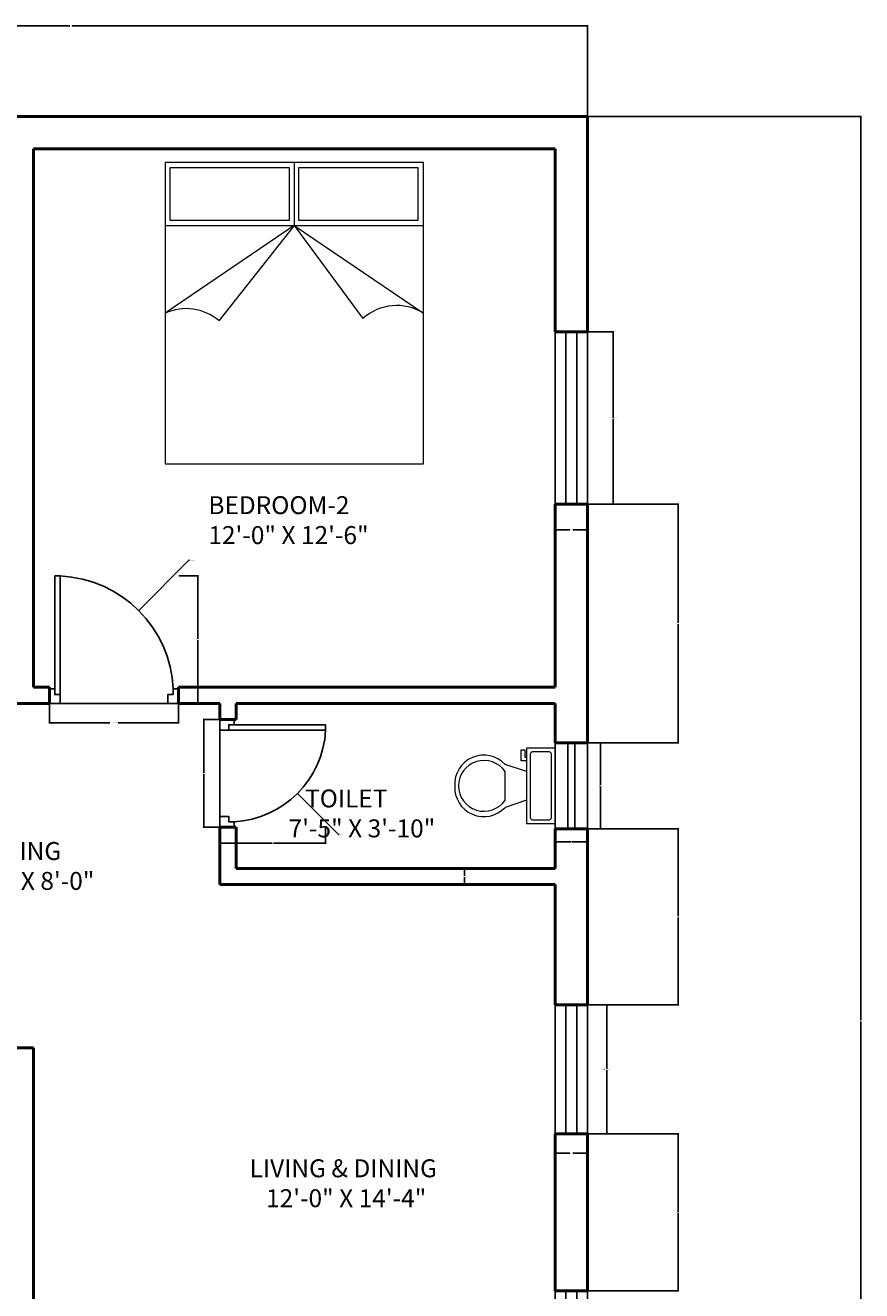
# Model space of a CAD drawing. Units: inches. Extents: x 17078 to 17468, y 5298 to 5853.
# Tile 3 of 3: x 17235 to 17468, y 5500 to 5853. Entities that reach past the tile are written whole.
import ezdxf

# ---------------------------------------------------------------- set-up
doc = ezdxf.new("R2010")
doc.units = ezdxf.units.IN
for name, color, linetype, lineweight in [('A-ANNO-DIMS', 2, 'Continuous', 18), ('A-AREA-IDEN', 7, 'Continuous', 18), ('A-FLOR-FIXT', 9, 'Continuous', 18), ('door', 30, 'Continuous', 25), ('furniture', 9, 'Continuous', 18), ('ventilator', 191, 'Continuous', 25), ('wall', 7, 'Continuous', 50), ('window1', 151, 'Continuous', 25)]:
    doc.layers.add(name, color=color, linetype=linetype, lineweight=lineweight)
doc.styles.get("Standard").update_dxf_attribs({"font": 'arial.ttf'})
doc.dimstyles.get("Standard").update_dxf_attribs({"dimtxt": 0.18, "dimasz": 0.18, "dimexe": 0.18, "dimexo": 0.0625, "dimgap": 0.09, "dimtad": 0, "dimtih": 1, "dimtoh": 1, "dimdec": 4, "dimzin": 0, "dimdsep": 46, "dimtxsty": 'Standard', "dimcen": 0.09, "dimadec": 0, "dimazin": 0, "dimtfac": 1, "dimtdec": 4, "dimtofl": 0, "dimtmove": 0, "dimatfit": 3, "dimfxl": 1, "dimtolj": 1, "dimtzin": 0, "dimarcsym": 0})

# ---------------------------------------------------------------- blocks, each defined once
blk = doc.blocks.new('d1')
at = {"layer": 'door'}
blk.add_line((17631.7, 5593.67), (17667.7, 5593.67), dxfattribs=at)
blk.add_lwpolyline([(17633.2, 5596.17), (17634.7, 5596.17), (17634.7, 5629.17), (17633.2, 5629.17)], close=True, dxfattribs=at)
for points in [[(17634.7, 5593.67), (17631.7, 5593.67), (17631.7, 5597.67), (17633.2, 5597.67), (17633.2, 5596.17), (17634.7, 5596.17), (17634.7, 5593.67)], [(17664.7, 5593.67), (17667.7, 5593.67), (17667.7, 5597.67), (17666.2, 5597.67), (17666.2, 5596.17), (17664.7, 5596.17), (17664.7, 5593.67)]]:
    blk.add_lwpolyline(points, dxfattribs=at)
blk.add_arc((17633.2, 5596.17), 33.03, 2.6026, 87.3974, dxfattribs=at)
blk = doc.blocks.new('d2')
at = {"layer": 'door'}
blk.add_line((17631.7, 5527.56), (17661.7, 5527.56), dxfattribs=at)
blk.add_lwpolyline([(17633.2, 5530.06), (17634.7, 5530.06), (17634.7, 5557.06), (17633.2, 5557.06)], close=True, dxfattribs=at)
for points in [[(17634.7, 5527.56), (17631.7, 5527.56), (17631.7, 5531.56), (17633.2, 5531.56), (17633.2, 5530.06), (17634.7, 5530.06), (17634.7, 5527.56)], [(17658.7, 5527.56), (17661.7, 5527.56), (17661.7, 5531.56), (17660.2, 5531.56), (17660.2, 5530.06), (17658.7, 5530.06), (17658.7, 5527.56)]]:
    blk.add_lwpolyline(points, dxfattribs=at)
blk.add_arc((17633.2, 5530.06), 27.04, 3.1798, 86.8202, dxfattribs=at)
blk = doc.blocks.new('w1')
at = {"layer": 'window1'}
for p, q in [((17477.6, 5616.65), (17477.6, 5580.65)), ((17480.6, 5616.65), (17480.6, 5580.65))]:
    blk.add_line(p, q, dxfattribs=at)
blk.add_lwpolyline([(17474.6, 5580.65), (17483.6, 5580.65), (17483.6, 5616.65), (17474.6, 5616.65)], close=True, dxfattribs=at)
blk = doc.blocks.new('v')
at = {"layer": 'ventilator'}
for p, q in [((17450.03, 5790.51), (17450.03, 5766.51)), ((17452.03, 5790.51), (17452.03, 5766.51))]:
    blk.add_line(p, q, dxfattribs=at)
blk.add_lwpolyline([(17446.53, 5766.51), (17455.53, 5766.51), (17455.53, 5790.51), (17446.53, 5790.51)], close=True, dxfattribs=at)
blk = doc.blocks.new('w2')
at = {"layer": 'window1'}
for p, q in [((17539.72, 5675.98), (17539.72, 5627.98)), ((17542.72, 5675.98), (17542.72, 5627.98))]:
    blk.add_line(p, q, dxfattribs=at)
blk.add_lwpolyline([(17536.72, 5627.98), (17545.72, 5627.98), (17545.72, 5675.98), (17536.72, 5675.98)], close=True, dxfattribs=at)
blk = doc.blocks.new('BED')
at = {"layer": 'furniture'}
for p, q in [((17631.72, 5825.16), (17631.72, 5807.64)), ((17595.72, 5807.64), (17667.72, 5807.64)), ((17631.72, 5807.64), (17595.72, 5783.16)), ((17631.72, 5807.64), (17610.71, 5781.09)), ((17631.72, 5807.64), (17667.72, 5783.16)), ((17631.72, 5807.64), (17650.87, 5781.67))]:
    blk.add_line(p, q, dxfattribs=at)
for points in [[(17595.72, 5741.16), (17667.72, 5741.16), (17667.72, 5825.16), (17595.72, 5825.16)], [(17597.14, 5823.74), (17630.27, 5823.74), (17630.27, 5809), (17597.14, 5809)], [(17633.01, 5823.74), (17666.14, 5823.74), (17666.14, 5809), (17633.01, 5809)]]:
    blk.add_lwpolyline(points, close=True, dxfattribs=at)
for centre, radius, start, end in [((17601.58, 5770.29), 14.15, 49.7949, 114.4561), ((17660.27, 5771.38), 13.94, 57.7012, 132.4176)]:
    blk.add_arc(centre, radius, start, end, dxfattribs=at)
blk = doc.blocks.new('*U8')
for p, q in [((241.3, -152.4), (241.3, -50.8)), ((-254, -215.9), (-203.2, -215.9)), ((-254, -241.3), (-254, -215.9)), ((-177.8, -241.3), (-254, -241.3)), ((-203.2, -215.9), (-203.2, -203.2)), ((-177.8, -203.2), (-177.8, -241.3)), ((-101.6, -203.2), (-152.4, -355.6)), ((101.6, -203.2), (152.4, -355.6)), ((101.6, -355.6), (-101.6, -355.6))]:
    blk.add_line(p, q)
blk.add_lwpolyline([(266.7, -203.2), (266.7, 0), (-266.7, 0), (-266.7, -203.2)], close=True)
for points in [[(-241.3, -50.8), (-241.3, -152.4)], [(215.9, -25.4), (-215.9, -25.4)], [(-215.9, -177.8), (215.9, -177.8)]]:
    blk.add_lwpolyline(points)
for centre, radius, start, end in [((-219.075, -47.625), 22.45064, 81.8699, 188.1301), ((219.075, -47.625), 22.45064, 351.8699, 98.1301), ((-219.075, -155.575), 22.45064, 171.869898, 278.1301), ((219.075, -155.575), 22.45064, 261.8699, 8.1301), ((-12.12088, -505.93752), 205.61935, 133.01722, 273.38), ((0.94996, -504.77674), 181.02486, 124.50543, 269.7), ((-0.94742, -504.77674), 181.02486, 270.3, 55.4946), ((12.12342, -505.93752), 205.61935, 266.62, 46.9828)]:
    blk.add_arc(centre, radius, start, end)
blk = doc.blocks.new('*D9')
at = {"layer": 'A-ANNO-DIMS', "color": 0, "lineweight": -2, "transparency": 16777216}
for p, q in [((17241.53, 5663.96), (17241.53, 5658.44)), ((17277.53, 5663.96), (17277.53, 5658.44)), ((17241.71, 5658.62), (17258.4, 5658.62)), ((17277.35, 5658.62), (17260.67, 5658.62))]:
    blk.add_line(p, q, dxfattribs=at)
at = {"layer": 'A-ANNO-DIMS', "color": 0, "transparency": 16777216}
for points in [[(17241.71, 5658.65), (17241.71, 5658.59), (17241.53, 5658.62)], [(17277.35, 5658.65), (17277.35, 5658.59), (17277.53, 5658.62)]]:
    blk.add_solid(points, dxfattribs=at)
at = {"layer": 'Defpoints', "color": 0, "transparency": 16777216}
for p in [(17241.53, 5664.02), (17277.53, 5664.02), (17277.53, 5658.62)]:
    blk.add_point(p, dxfattribs=at)
at = {"layer": 'A-ANNO-DIMS', "color": 0, "transparency": 16777216, "insert": (17259.53, 5658.62), "char_height": 0.18, "attachment_point": 5}
blk.add_mtext('\\A1;DOOR D1 36 TYP.', dxfattribs=at)
blk = doc.blocks.new('*D10')
at = {"layer": 'A-ANNO-DIMS', "color": 0, "lineweight": -2, "transparency": 16777216}
for p, q in [((17277.6, 5699.52), (17283.11, 5699.52)), ((17282.93, 5699.34), (17282.93, 5681.95)), ((17282.93, 5664.2), (17282.93, 5681.59)), ((17277.6, 5664.02), (17283.11, 5664.02))]:
    blk.add_line(p, q, dxfattribs=at)
at = {"layer": 'A-ANNO-DIMS', "color": 0, "transparency": 16777216}
for points in [[(17282.9, 5699.34), (17282.96, 5699.34), (17282.93, 5699.52)], [(17282.9, 5664.2), (17282.96, 5664.2), (17282.93, 5664.02)]]:
    blk.add_solid(points, dxfattribs=at)
at = {"layer": 'Defpoints', "color": 0, "transparency": 16777216}
for p in [(17277.53, 5699.52), (17282.93, 5699.52), (17277.53, 5664.02)]:
    blk.add_point(p, dxfattribs=at)
at = {"layer": 'A-ANNO-DIMS', "color": 0, "transparency": 16777216, "insert": (17282.93, 5681.77), "char_height": 0.18, "attachment_point": 5}
blk.add_mtext('\\A1;36 TYP.', dxfattribs=at)
blk = doc.blocks.new('*D11')
at = {"layer": 'A-ANNO-DIMS', "color": 0, "lineweight": -2, "transparency": 16777216}
for p, q in [((17288.97, 5659.52), (17284.35, 5659.52)), ((17284.53, 5659.34), (17284.53, 5644.7)), ((17284.53, 5629.7), (17284.53, 5644.34)), ((17288.97, 5629.52), (17284.35, 5629.52))]:
    blk.add_line(p, q, dxfattribs=at)
at = {"layer": 'A-ANNO-DIMS', "color": 0, "transparency": 16777216}
for points in [[(17284.5, 5659.34), (17284.56, 5659.34), (17284.53, 5659.52)], [(17284.5, 5629.7), (17284.56, 5629.7), (17284.53, 5629.52)]]:
    blk.add_solid(points, dxfattribs=at)
at = {"layer": 'Defpoints', "color": 0, "transparency": 16777216}
for p in [(17289.03, 5659.52), (17284.53, 5629.52), (17289.03, 5629.52)]:
    blk.add_point(p, dxfattribs=at)
at = {"layer": 'A-ANNO-DIMS', "color": 0, "transparency": 16777216, "insert": (17284.53, 5644.52), "char_height": 0.18, "attachment_point": 5}
blk.add_mtext('\\A1;DOOR D2 30', dxfattribs=at)
blk = doc.blocks.new('*D12')
at = {"layer": 'A-ANNO-DIMS', "color": 0, "lineweight": -2, "transparency": 16777216}
for p, q in [((17289.03, 5629.46), (17289.03, 5624.84)), ((17318.53, 5629.46), (17318.53, 5624.84)), ((17289.21, 5625.02), (17303.57, 5625.02)), ((17318.35, 5625.02), (17304, 5625.02))]:
    blk.add_line(p, q, dxfattribs=at)
at = {"layer": 'A-ANNO-DIMS', "color": 0, "transparency": 16777216}
for points in [[(17289.21, 5625.05), (17289.21, 5624.99), (17289.03, 5625.02)], [(17318.35, 5625.05), (17318.35, 5624.99), (17318.53, 5625.02)]]:
    blk.add_solid(points, dxfattribs=at)
at = {"layer": 'Defpoints', "color": 0, "transparency": 16777216}
for p in [(17289.03, 5629.52), (17318.53, 5629.52), (17318.53, 5625.02)]:
    blk.add_point(p, dxfattribs=at)
at = {"layer": 'A-ANNO-DIMS', "color": 0, "transparency": 16777216, "insert": (17303.78, 5625.02), "char_height": 0.18, "attachment_point": 5}
blk.add_mtext('\\A1;30', dxfattribs=at)
blk = doc.blocks.new('*D13')
at = {"layer": 'A-ANNO-DIMS', "color": 0, "lineweight": -2, "transparency": 16777216}
for p, q in [((17391.6, 5767.52), (17398.91, 5767.52)), ((17398.73, 5767.34), (17398.73, 5743.7)), ((17398.73, 5719.7), (17398.73, 5743.34)), ((17391.6, 5719.52), (17398.91, 5719.52))]:
    blk.add_line(p, q, dxfattribs=at)
at = {"layer": 'A-ANNO-DIMS', "color": 0, "transparency": 16777216}
for points in [[(17398.7, 5767.34), (17398.76, 5767.34), (17398.73, 5767.52)], [(17398.7, 5719.7), (17398.76, 5719.7), (17398.73, 5719.52)]]:
    blk.add_solid(points, dxfattribs=at)
at = {"layer": 'Defpoints', "color": 0, "transparency": 16777216}
for p in [(17391.53, 5767.52), (17398.73, 5767.52), (17391.53, 5719.52)]:
    blk.add_point(p, dxfattribs=at)
at = {"layer": 'A-ANNO-DIMS', "color": 0, "transparency": 16777216, "insert": (17398.73, 5743.52), "char_height": 0.18, "attachment_point": 5}
blk.add_mtext('\\A1;WINDOW W2 48 TYP.', dxfattribs=at)
blk = doc.blocks.new('*D14')
at = {"layer": 'A-ANNO-DIMS', "color": 0, "lineweight": -2, "transparency": 16777216}
for p, q in [((17382.53, 5719.46), (17382.53, 5712.14)), ((17391.53, 5719.46), (17391.53, 5712.14)), ((17382.71, 5712.32), (17386.58, 5712.32)), ((17391.35, 5712.32), (17387.49, 5712.32))]:
    blk.add_line(p, q, dxfattribs=at)
at = {"layer": 'A-ANNO-DIMS', "color": 0, "transparency": 16777216}
for points in [[(17382.71, 5712.35), (17382.71, 5712.29), (17382.53, 5712.32)], [(17391.35, 5712.35), (17391.35, 5712.29), (17391.53, 5712.32)]]:
    blk.add_solid(points, dxfattribs=at)
at = {"layer": 'Defpoints', "color": 0, "transparency": 16777216}
for p in [(17382.53, 5719.52), (17391.53, 5719.52), (17391.53, 5712.32)]:
    blk.add_point(p, dxfattribs=at)
at = {"layer": 'A-ANNO-DIMS', "color": 0, "transparency": 16777216, "insert": (17387.03, 5712.32), "char_height": 0.18, "attachment_point": 5}
blk.add_mtext('\\A1;9 TYP.', dxfattribs=at)
blk = doc.blocks.new('*D15')
at = {"layer": 'A-ANNO-DIMS', "color": 0, "lineweight": -2, "transparency": 16777216}
for p, q in [((17391.6, 5580.03), (17397.11, 5580.03)), ((17396.93, 5579.85), (17396.93, 5562.21)), ((17396.93, 5544.21), (17396.93, 5561.84)), ((17391.6, 5544.03), (17397.11, 5544.03))]:
    blk.add_line(p, q, dxfattribs=at)
at = {"layer": 'A-ANNO-DIMS', "color": 0, "transparency": 16777216}
for points in [[(17396.9, 5579.85), (17396.96, 5579.85), (17396.93, 5580.03)], [(17396.9, 5544.21), (17396.96, 5544.21), (17396.93, 5544.03)]]:
    blk.add_solid(points, dxfattribs=at)
at = {"layer": 'Defpoints', "color": 0, "transparency": 16777216}
for p in [(17391.53, 5580.03), (17396.93, 5580.03), (17391.53, 5544.03)]:
    blk.add_point(p, dxfattribs=at)
at = {"layer": 'A-ANNO-DIMS', "color": 0, "transparency": 16777216, "insert": (17396.93, 5562.03), "char_height": 0.18, "attachment_point": 5}
blk.add_mtext('\\A1;WINDOW W1 36 TYP.', dxfattribs=at)
blk = doc.blocks.new('*D16')
at = {"layer": 'A-ANNO-DIMS', "color": 0, "lineweight": -2, "transparency": 16777216}
for p, q in [((17382.53, 5543.96), (17382.53, 5538.45)), ((17391.53, 5543.96), (17391.53, 5538.45)), ((17382.71, 5538.63), (17386.58, 5538.63)), ((17391.35, 5538.63), (17387.49, 5538.63))]:
    blk.add_line(p, q, dxfattribs=at)
at = {"layer": 'A-ANNO-DIMS', "color": 0, "transparency": 16777216}
for points in [[(17382.71, 5538.66), (17382.71, 5538.6), (17382.53, 5538.63)], [(17391.35, 5538.66), (17391.35, 5538.6), (17391.53, 5538.63)]]:
    blk.add_solid(points, dxfattribs=at)
at = {"layer": 'Defpoints', "color": 0, "transparency": 16777216}
for p in [(17382.53, 5544.03), (17391.53, 5544.03), (17391.53, 5538.63)]:
    blk.add_point(p, dxfattribs=at)
at = {"layer": 'A-ANNO-DIMS', "color": 0, "transparency": 16777216, "insert": (17387.03, 5538.63), "char_height": 0.18, "attachment_point": 5}
blk.add_mtext('\\A1;9 TYP.', dxfattribs=at)
blk = doc.blocks.new('*D17')
at = {"layer": 'A-ANNO-DIMS', "color": 0, "lineweight": -2, "transparency": 16777216}
for p, q in [((17391.6, 5653.02), (17395.31, 5653.02)), ((17395.13, 5652.84), (17395.13, 5641.2)), ((17395.13, 5629.2), (17395.13, 5640.84)), ((17391.6, 5629.02), (17395.31, 5629.02))]:
    blk.add_line(p, q, dxfattribs=at)
at = {"layer": 'A-ANNO-DIMS', "color": 0, "transparency": 16777216}
for points in [[(17395.1, 5652.84), (17395.16, 5652.84), (17395.13, 5653.02)], [(17395.1, 5629.2), (17395.16, 5629.2), (17395.13, 5629.02)]]:
    blk.add_solid(points, dxfattribs=at)
at = {"layer": 'Defpoints', "color": 0, "transparency": 16777216}
for p in [(17391.53, 5653.02), (17395.13, 5653.02), (17391.53, 5629.02)]:
    blk.add_point(p, dxfattribs=at)
at = {"layer": 'A-ANNO-DIMS', "color": 0, "transparency": 16777216, "insert": (17395.13, 5641.02), "char_height": 0.18, "attachment_point": 5}
blk.add_mtext('\\A1;VENT 24', dxfattribs=at)
blk = doc.blocks.new('*D18')
at = {"layer": 'A-ANNO-DIMS', "color": 0, "lineweight": -2, "transparency": 16777216}
for p, q in [((17382.53, 5628.96), (17382.53, 5625.24)), ((17391.53, 5628.96), (17391.53, 5625.24)), ((17382.71, 5625.42), (17386.88, 5625.42)), ((17391.35, 5625.42), (17387.18, 5625.42))]:
    blk.add_line(p, q, dxfattribs=at)
at = {"layer": 'A-ANNO-DIMS', "color": 0, "transparency": 16777216}
for points in [[(17382.71, 5625.45), (17382.71, 5625.39), (17382.53, 5625.42)], [(17391.35, 5625.45), (17391.35, 5625.39), (17391.53, 5625.42)]]:
    blk.add_solid(points, dxfattribs=at)
at = {"layer": 'Defpoints', "color": 0, "transparency": 16777216}
for p in [(17382.53, 5629.02), (17391.53, 5629.02), (17391.53, 5625.42)]:
    blk.add_point(p, dxfattribs=at)
at = {"layer": 'A-ANNO-DIMS', "color": 0, "transparency": 16777216, "insert": (17387.03, 5625.42), "char_height": 0.18, "attachment_point": 5}
blk.add_mtext('\\A1;9', dxfattribs=at)
blk = doc.blocks.new('*D21')
at = {"layer": 'A-ANNO-DIMS', "color": 0, "lineweight": -2, "transparency": 16777216}
for p, q in [((17103.53, 5827.58), (17103.53, 5852.95)), ((17103.71, 5852.77), (17247.24, 5852.77)), ((17391.35, 5852.77), (17247.82, 5852.77)), ((17391.53, 5827.58), (17391.53, 5852.95))]:
    blk.add_line(p, q, dxfattribs=at)
at = {"layer": 'A-ANNO-DIMS', "color": 0, "transparency": 16777216}
for points in [[(17103.71, 5852.8), (17103.71, 5852.74), (17103.53, 5852.77)], [(17391.35, 5852.8), (17391.35, 5852.74), (17391.53, 5852.77)]]:
    blk.add_solid(points, dxfattribs=at)
at = {"layer": 'Defpoints', "color": 0, "transparency": 16777216}
for p in [(17391.53, 5852.77), (17103.53, 5827.52), (17391.53, 5827.52)]:
    blk.add_point(p, dxfattribs=at)
at = {"layer": 'A-ANNO-DIMS', "color": 0, "transparency": 16777216, "insert": (17247.53, 5852.77), "char_height": 0.18, "attachment_point": 5}
blk.add_mtext('\\A1;288', dxfattribs=at)
blk = doc.blocks.new('*D22')
at = {"layer": 'A-ANNO-DIMS', "color": 0, "lineweight": -2, "transparency": 16777216}
for p, q in [((17391.6, 5827.52), (17467.96, 5827.52)), ((17467.78, 5827.34), (17467.78, 5575.7)), ((17467.78, 5323.7), (17467.78, 5575.34)), ((17391.6, 5323.52), (17467.96, 5323.52))]:
    blk.add_line(p, q, dxfattribs=at)
at = {"layer": 'A-ANNO-DIMS', "color": 0, "transparency": 16777216}
for points in [[(17467.75, 5827.34), (17467.81, 5827.34), (17467.78, 5827.52)], [(17467.75, 5323.7), (17467.81, 5323.7), (17467.78, 5323.52)]]:
    blk.add_solid(points, dxfattribs=at)
at = {"layer": 'Defpoints', "color": 0, "transparency": 16777216}
for p in [(17391.53, 5827.52), (17467.78, 5827.52), (17391.53, 5323.52)]:
    blk.add_point(p, dxfattribs=at)
at = {"layer": 'A-ANNO-DIMS', "color": 0, "transparency": 16777216, "insert": (17467.78, 5575.52), "char_height": 0.18, "attachment_point": 5}
blk.add_mtext('\\A1;504', dxfattribs=at)
blk = doc.blocks.new('*D33')
at = {"layer": 'A-ANNO-DIMS', "color": 0, "lineweight": -2, "transparency": 16777216}
for p, q in [((17391.6, 5544.03), (17416.96, 5544.03)), ((17416.78, 5543.85), (17416.78, 5522.37)), ((17416.78, 5500.53), (17416.78, 5522.01)), ((17391.6, 5500.35), (17416.96, 5500.35))]:
    blk.add_line(p, q, dxfattribs=at)
at = {"layer": 'A-ANNO-DIMS', "color": 0, "transparency": 16777216}
for points in [[(17416.75, 5543.85), (17416.81, 5543.85), (17416.78, 5544.03)], [(17416.75, 5500.53), (17416.81, 5500.53), (17416.78, 5500.35)]]:
    blk.add_solid(points, dxfattribs=at)
at = {"layer": 'Defpoints', "color": 0, "transparency": 16777216}
for p in [(17391.53, 5544.03), (17391.53, 5500.35), (17416.78, 5500.35)]:
    blk.add_point(p, dxfattribs=at)
at = {"layer": 'A-ANNO-DIMS', "color": 0, "transparency": 16777216, "insert": (17416.78, 5522.19), "char_height": 0.18, "attachment_point": 5}
blk.add_mtext('\\A1;43.67', dxfattribs=at)
blk = doc.blocks.new('*D34')
at = {"layer": 'A-ANNO-DIMS', "color": 0, "lineweight": -2, "transparency": 16777216}
for p, q in [((17391.6, 5629.02), (17416.96, 5629.02)), ((17416.78, 5628.84), (17416.78, 5604.71)), ((17416.78, 5580.21), (17416.78, 5604.34)), ((17391.6, 5580.03), (17416.96, 5580.03))]:
    blk.add_line(p, q, dxfattribs=at)
at = {"layer": 'A-ANNO-DIMS', "color": 0, "transparency": 16777216}
for points in [[(17416.75, 5628.84), (17416.81, 5628.84), (17416.78, 5629.02)], [(17416.75, 5580.21), (17416.81, 5580.21), (17416.78, 5580.03)]]:
    blk.add_solid(points, dxfattribs=at)
at = {"layer": 'Defpoints', "color": 0, "transparency": 16777216}
for p in [(17391.53, 5629.02), (17391.53, 5580.03), (17416.78, 5580.03)]:
    blk.add_point(p, dxfattribs=at)
at = {"layer": 'A-ANNO-DIMS', "color": 0, "transparency": 16777216, "insert": (17416.78, 5604.52), "char_height": 0.18, "attachment_point": 5}
blk.add_mtext('\\A1;48.99', dxfattribs=at)
blk = doc.blocks.new('*D35')
at = {"layer": 'A-ANNO-DIMS', "color": 0, "lineweight": -2, "transparency": 16777216}
for p, q in [((17391.6, 5719.52), (17416.96, 5719.52)), ((17416.78, 5719.34), (17416.78, 5686.45)), ((17416.78, 5653.2), (17416.78, 5686.09)), ((17391.6, 5653.02), (17416.96, 5653.02))]:
    blk.add_line(p, q, dxfattribs=at)
at = {"layer": 'A-ANNO-DIMS', "color": 0, "transparency": 16777216}
for points in [[(17416.75, 5719.34), (17416.81, 5719.34), (17416.78, 5719.52)], [(17416.75, 5653.2), (17416.81, 5653.2), (17416.78, 5653.02)]]:
    blk.add_solid(points, dxfattribs=at)
at = {"layer": 'Defpoints', "color": 0, "transparency": 16777216}
for p in [(17391.53, 5719.52), (17391.53, 5653.02), (17416.78, 5653.02)]:
    blk.add_point(p, dxfattribs=at)
at = {"layer": 'A-ANNO-DIMS', "color": 0, "transparency": 16777216, "insert": (17416.78, 5686.27), "char_height": 0.18, "attachment_point": 5}
blk.add_mtext('\\A1;66.5', dxfattribs=at)
blk = doc.blocks.new('*D36')
at = {"layer": 'A-ANNO-DIMS', "color": 0, "lineweight": -2, "transparency": 16777216}
for p, q in [((17382.47, 5618.02), (17357.1, 5618.02)), ((17357.28, 5617.84), (17357.28, 5615.95)), ((17382.47, 5613.52), (17357.1, 5613.52)), ((17357.28, 5613.7), (17357.28, 5615.59))]:
    blk.add_line(p, q, dxfattribs=at)
at = {"layer": 'A-ANNO-DIMS', "color": 0, "transparency": 16777216}
for points in [[(17357.25, 5617.84), (17357.31, 5617.84), (17357.28, 5618.02)], [(17357.25, 5613.7), (17357.31, 5613.7), (17357.28, 5613.52)]]:
    blk.add_solid(points, dxfattribs=at)
at = {"layer": 'Defpoints', "color": 0, "transparency": 16777216}
for p in [(17357.28, 5618.02), (17382.53, 5618.02), (17382.53, 5613.52)]:
    blk.add_point(p, dxfattribs=at)
at = {"layer": 'A-ANNO-DIMS', "color": 0, "transparency": 16777216, "insert": (17357.28, 5615.77), "char_height": 0.18, "attachment_point": 5}
blk.add_mtext('\\A1;4.5', dxfattribs=at)
blk = doc.blocks.new('*D43')
at = {"layer": 'A-ANNO-DIMS', "color": 0, "lineweight": -2, "transparency": 16777216}
for p, q in [((17280.41, 5703.89), (17266.52, 5690.01)), ((17280.59, 5703.89), (17280.41, 5703.89)), ((17242.94, 5666.52), (17243.12, 5666.52)), ((17243.03, 5666.43), (17243.03, 5666.61))]:
    blk.add_line(p, q, dxfattribs=at)
at = {"layer": 'A-ANNO-DIMS', "color": 0, "transparency": 16777216}
blk.add_solid([(17266.5, 5690.03), (17266.54, 5689.98), (17266.39, 5689.88)], dxfattribs=at)
at = {"layer": 'Defpoints', "color": 0, "transparency": 16777216}
for p in [(17266.39, 5689.88), (17243.03, 5666.52)]:
    blk.add_point(p, dxfattribs=at)
at = {"layer": 'A-ANNO-DIMS', "color": 0, "transparency": 16777216, "insert": (17281.33, 5703.89), "char_height": 0.18, "attachment_point": 5}
blk.add_mtext('\\A1;4X R33.034', dxfattribs=at)
blk = doc.blocks.new('*D44')
at = {"layer": 'A-ANNO-DIMS', "color": 0, "lineweight": -2, "transparency": 16777216}
for p, q in [((17291.44, 5658.02), (17291.62, 5658.02)), ((17291.53, 5657.93), (17291.53, 5658.11)), ((17322.13, 5627.43), (17310.78, 5638.77)), ((17322.31, 5627.43), (17322.13, 5627.43))]:
    blk.add_line(p, q, dxfattribs=at)
at = {"layer": 'A-ANNO-DIMS', "color": 0, "transparency": 16777216}
blk.add_solid([(17310.8, 5638.79), (17310.76, 5638.75), (17310.66, 5638.9)], dxfattribs=at)
at = {"layer": 'Defpoints', "color": 0, "transparency": 16777216}
for p in [(17291.53, 5658.02), (17310.66, 5638.9)]:
    blk.add_point(p, dxfattribs=at)
at = {"layer": 'A-ANNO-DIMS', "color": 0, "transparency": 16777216, "insert": (17322.79, 5627.43), "char_height": 0.18, "attachment_point": 5}
blk.add_mtext('\\A1;R27.04', dxfattribs=at)

msp = doc.modelspace()

# ---------------------------------------------------------------- linework, layer by layer
at = {"layer": 'wall'}
for p, q in [((17391.534, 5827.52), (17103.534, 5827.52)), ((17391.534, 5767.52), (17391.534, 5827.52)), ((17382.534, 5818.52), (17237.034, 5818.52)), ((17237.034, 5818.52), (17237.034, 5668.52)), ((17382.534, 5767.52), (17382.534, 5818.52)), ((17382.534, 5767.52), (17391.534, 5767.52)), ((17382.534, 5668.52), (17382.534, 5719.52)), ((17382.534, 5719.52), (17391.534, 5719.52)), ((17391.534, 5653.02), (17391.534, 5719.52)), ((17241.534, 5668.52), (17237.034, 5668.52)), ((17241.534, 5668.52), (17241.534, 5664.02)), ((17382.534, 5668.52), (17277.534, 5668.52)), ((17277.534, 5668.52), (17277.534, 5664.02)), ((17241.534, 5664.02), (17228.034, 5664.02)), ((17289.034, 5664.02), (17277.534, 5664.02)), ((17289.034, 5659.52), (17289.034, 5664.02)), ((17382.534, 5664.02), (17293.534, 5664.02)), ((17293.534, 5659.52), (17293.534, 5664.02)), ((17382.534, 5653.02), (17382.534, 5664.02)), ((17293.534, 5659.52), (17289.034, 5659.52)), ((17382.534, 5653.02), (17391.534, 5653.02)), ((17289.034, 5613.52), (17289.034, 5629.52)), ((17293.534, 5629.52), (17289.034, 5629.52)), ((17293.534, 5618.02), (17293.534, 5629.52)), ((17382.534, 5618.02), (17382.534, 5629.02)), ((17382.534, 5629.02), (17391.534, 5629.02)), ((17391.534, 5580.0271), (17391.534, 5629.02)), ((17382.534, 5618.02), (17293.534, 5618.02)), ((17382.534, 5613.52), (17289.034, 5613.52)), ((17382.534, 5580.0271), (17382.534, 5613.52)), ((17382.534, 5580.0271), (17391.534, 5580.0271)), ((17237.034, 5568.02), (17228.034, 5568.02)), ((17237.034, 5568.02), (17237.034, 5442.52)), ((17382.534, 5544.0271), (17391.534, 5544.0271)), ((17382.534, 5500.3549), (17382.534, 5544.0271)), ((17391.534, 5500.3549), (17391.534, 5544.0271)), ((17382.534, 5500.3549), (17391.534, 5500.3549))]:
    msp.add_line(p, q, dxfattribs=at)

# ---------------------------------------------------------------- block references
at = {"layer": 'A-FLOR-FIXT', "xscale": 0.0393700787401575, "yscale": 0.0393700787401575, "zscale": 0.0393700787401575, "rotation": 270}
msp.add_blockref('*U8', (17382.534, 5641.02), dxfattribs=at)
at = {"layer": 'door'}
msp.add_blockref('d1', (-390.1629, 70.3471), dxfattribs=at)
at = {"layer": 'door', "rotation": 270}
msp.add_blockref('d2', (11761.4695, 23291.2169), dxfattribs=at)
at = {"layer": 'furniture'}
msp.add_blockref('BED', (-321.936, -10.4456), dxfattribs=at)
at = {"layer": 'ventilator'}
msp.add_blockref('v', (-63.9998, -137.4916), dxfattribs=at)
at = {"layer": 'window1'}
for name, p in [('w2', (-154.1828, 91.541)), ('w1', (-92.0702, -36.6261)), ('w1', (-92.0702, -116.2984))]:
    msp.add_blockref(name, p, dxfattribs=at)

# ---------------------------------------------------------------- texts
at = {"layer": 'A-AREA-IDEN', "char_height": 5, "attachment_point": 1}
for s, width, insert in [('BEDROOM-2\\P12\'-0" X 12\'-6"', 48.964, (17285.8311, 5721.7395)), ('   TOILET\\P7\'-5" X 3\'-10"', 48.964, (17308.2073, 5640.0062)), ('   DINING\\P8\'-1" X 8\'-0"', 48.964, (17216.9513, 5625.3725)), ('LIVING & DINING\\P   12\'-0" X 14\'-4"', 60.242862, (17297.3383, 5536.9605))]:
    msp.add_mtext_dynamic_manual_height_columns(s, width=width, gutter_width=12.5, heights=[0], dxfattribs=dict(at, insert=insert))

# ---------------------------------------------------------------- dimensions: what is measured, and where the dimension line sits
at = {"layer": 'A-ANNO-DIMS'}
for base, p1, p2, picture, middle in [((17391.534, 5852.77), (17103.534, 5827.52), (17391.534, 5827.52), '*D21', (17247.534, 5852.77)), ((17318.5340052605, 5625.0200193243), (17289.0340052605, 5629.5200193243), (17318.5340052605, 5629.5200193243), '*D12', (17303.7840052605, 5625.0200193243)), ((17391.534, 5625.42), (17382.534, 5629.02), (17391.534, 5629.02), '*D18', (17387.034, 5625.42))]:
    dim = msp.add_linear_dim(base=base, p1=p1, p2=p2, dimstyle='Standard', override={"dimdec": 0, "dimlfac": 1, "dimrnd": 0, "dimzin": 0, "dimdsep": 46, "dimlunit": 2}, dxfattribs=at)
    dim.commit()
    dim.dimension.update_dxf_attribs({"geometry": picture, "text_midpoint": middle})
for base, p1, p2, angle, override, picture, middle in [((17467.784, 5827.52), (17391.534, 5323.52), (17391.534, 5827.52), 90, {"dimdec": 0, "dimlfac": 1, "dimrnd": 0, "dimzin": 0, "dimdsep": 46, "dimlunit": 2}, '*D22', (17467.784, 5575.52)), ((17416.784, 5653.02), (17391.534, 5719.52), (17391.534, 5653.02), 270, {"dimdec": 1, "dimlfac": 1, "dimrnd": 0, "dimzin": 0, "dimdsep": 46, "dimlunit": 2}, '*D35', (17416.784, 5686.27)), ((17416.784, 5580.0271), (17391.534, 5629.02), (17391.534, 5580.0271), 270, {"dimdec": 2, "dimlfac": 1, "dimrnd": 0, "dimzin": 0, "dimdsep": 46, "dimlunit": 2}, '*D34', (17416.784, 5604.5236)), ((17357.284, 5618.02), (17382.534, 5613.52), (17382.534, 5618.02), 90, {"dimdec": 1, "dimlfac": 1, "dimrnd": 0, "dimzin": 0, "dimdsep": 46, "dimlunit": 2}, '*D36', (17357.284, 5615.77)), ((17416.784, 5500.3549), (17391.534, 5544.0271), (17391.534, 5500.3549), 270, {"dimdec": 2, "dimlfac": 1, "dimrnd": 0, "dimzin": 0, "dimdsep": 46, "dimlunit": 2}, '*D33', (17416.784, 5522.191))]:
    dim = msp.add_linear_dim(base=base, p1=p1, p2=p2, angle=angle, dimstyle='Standard', override=override, dxfattribs=at)
    dim.commit()
    dim.dimension.update_dxf_attribs({"geometry": picture, "text_midpoint": middle})
for base, p1, p2, angle, text, picture, middle in [((17398.734, 5767.52), (17391.534, 5719.52), (17391.534, 5767.52), 90, 'WINDOW W2 <> TYP.', '*D13', (17398.734, 5743.52)), ((17282.9340052605, 5699.5200193243), (17277.5340052605, 5664.0200193243), (17277.5340052605, 5699.5200193243), 90, '<> TYP.', '*D10', (17282.9340052605, 5681.7700193243)), ((17284.534, 5629.52), (17289.034, 5659.52), (17289.034, 5629.52), 270, 'DOOR D2 <>', '*D11', (17284.534, 5644.52)), ((17395.134, 5653.02), (17391.534, 5629.02), (17391.534, 5653.02), 90, 'VENT <>', '*D17', (17395.134, 5641.02)), ((17396.934, 5580.0271), (17391.534, 5544.0271), (17391.534, 5580.0271), 90, 'WINDOW W1 <> TYP.', '*D15', (17396.934, 5562.0271))]:
    dim = msp.add_linear_dim(base=base, p1=p1, p2=p2, angle=angle, text=text, dimstyle='Standard', override={"dimdec": 0, "dimlfac": 1, "dimrnd": 0, "dimzin": 0, "dimdsep": 46, "dimlunit": 2}, dxfattribs=at)
    dim.commit()
    dim.dimension.update_dxf_attribs({"geometry": picture, "text_midpoint": middle})
for base, p1, p2, text, picture, middle in [((17391.534, 5712.32), (17382.534, 5719.52), (17391.534, 5719.52), '<> TYP.', '*D14', (17387.034, 5712.32)), ((17277.534, 5658.62), (17241.534, 5664.02), (17277.534, 5664.02), 'DOOR D1 <> TYP.', '*D9', (17259.534, 5658.62)), ((17391.534, 5538.6271), (17382.534, 5544.0271), (17391.534, 5544.0271), '<> TYP.', '*D16', (17387.034, 5538.6271))]:
    dim = msp.add_linear_dim(base=base, p1=p1, p2=p2, text=text, dimstyle='Standard', override={"dimdec": 0, "dimlfac": 1, "dimrnd": 0, "dimzin": 0, "dimdsep": 46, "dimlunit": 2}, dxfattribs=at)
    dim.commit()
    dim.dimension.update_dxf_attribs({"geometry": picture, "text_midpoint": middle})
dim = msp.add_radius_dim(center=(17243.034, 5666.52), mpoint=(17266.3926, 5689.8786), text='4X <>', dimstyle='Standard', override={"dimdec": 3, "dimlfac": 1, "dimrnd": 0, "dimzin": 0, "dimdsep": 46, "dimlunit": 2}, dxfattribs=at)
dim.commit()
dim.dimension.update_dxf_attribs({"geometry": '*D43', "text_midpoint": (17281.3342, 5703.8938), "dimtype": 164})
dim = msp.add_radius_dim(center=(17291.534, 5658.02), mpoint=(17310.6553, 5638.8987), dimstyle='Standard', override={"dimdec": 2, "dimlfac": 1, "dimrnd": 0, "dimzin": 0, "dimdsep": 46, "dimlunit": 2}, dxfattribs=at)
dim.commit()
dim.dimension.update_dxf_attribs({"geometry": '*D44', "text_midpoint": (17322.7876, 5627.4259), "dimtype": 164})

doc.saveas('drawing.dxf')
